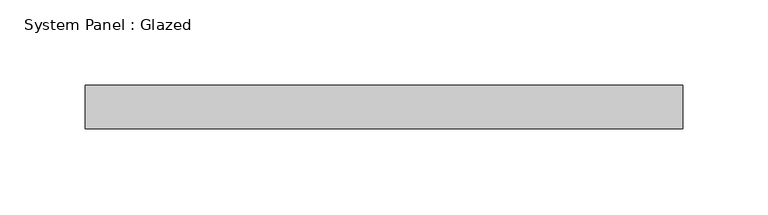
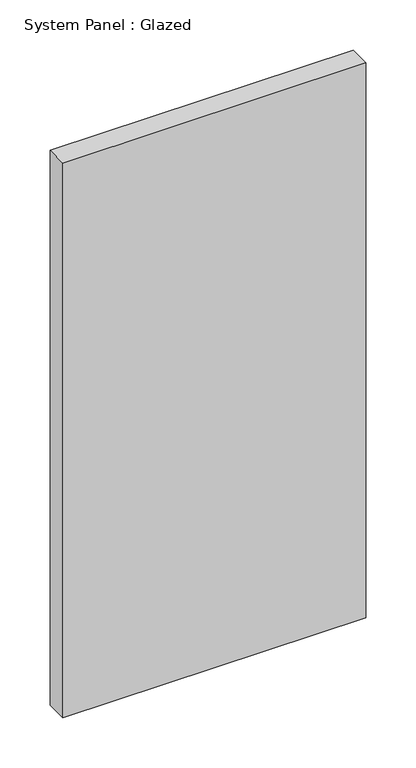
"""IFC4 building model written with IfcOpenShell, lengths in millimetres: plate geometry, System Panel : Glazed."""

from ifc_helpers import new_model, si_unit, origin, origin_with_axes, place, context, project, spatial, polyline, outline, extrude, source, transform, mapped, element, save


def system_panel_glazed_04b6ff1d(model_context):
    return source(origin(), model_context, "Body", "SweptSolid", [
        extrude(outline(polyline([(174.625, 19.05), (-174.625, 19.05), (-174.625, 44.45), (174.625, 44.45), (174.625, 19.05)])), origin_with_axes(), (0.0, 0.0, 1.0), 676.335164),
    ])


if __name__ == "__main__":
    model = new_model("IFC4")
    model_context = context("Model", 3, world=origin())
    ifc_project = project(units=[si_unit("LENGTHUNIT", "METRE", prefix="MILLI")], contexts=[model_context])
    site = spatial("IfcSite", under=ifc_project)
    building = spatial("IfcBuilding", under=site)
    placement = place(None, origin())
    system_panel_glazed_shape = system_panel_glazed_04b6ff1d(model_context)
    element("IfcPlate", 1, ObjectType="System Panel : Glazed", at=placement, inside=building, context=model_context, shape_type="MappedRepresentation", body=[
        mapped(system_panel_glazed_shape, transform((0.0, 0.0, 0.0), x_axis=(1.0, 0.0, 0.0), y_axis=(0.0, 1.0, 0.0), z_axis=(0.0, 0.0, 1.0))),
    ])
    save(model, "model.ifc")

# Revit data of these elements
# Type "System Panel : Glazed"
#   Construction Type Id = "GSP4R"
#   Analytic Construction = "1/8 in Pilkington single glazing"
#   Visual Light Transmittance = 0.9
#   Solar Heat Gain Coefficient = 0.86
#   Heat Transfer Coefficient (U) = 1.18115 BTU/(h·ft²·°F)
#   Define Thermal Properties by = 1
# Element 1 (IfcPlate, "System Panel : Glazed")
#   Materials on its faces: "Glass"
# Materials
#   "Glass": class "Glass", colour RGB 0 128 192, transparency 0.75, Description = "Soda Lime Glass", Cost = 0
